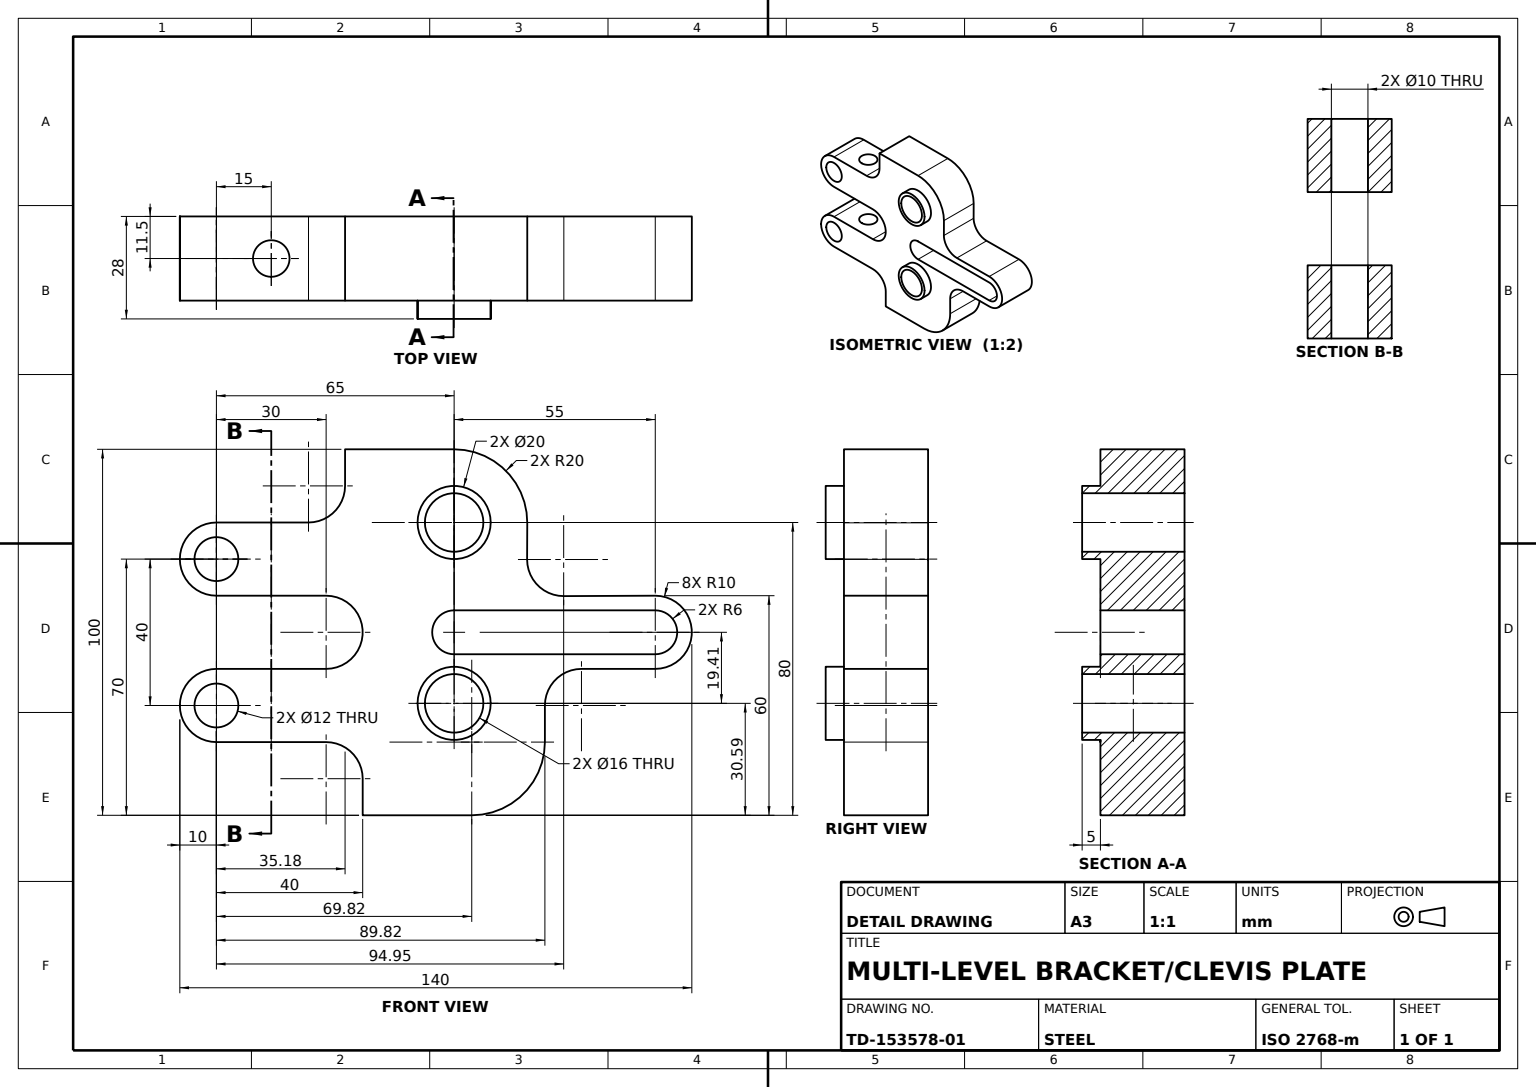
from build123d import *

# Parameters (mm, degrees)
BRACKET_PROFILE_SKETCH_R = 6
BRACKET_BASE_23MM_DEPTH  = 23
BOSS_PAD_SKETCH_R        = 10
BOSS_PAD_SKETCH_R_2      = 8
BOSS_PAD_5MM_DEPTH       = 5
HOLE_10_SKETCH_R         = 5
HOLE_10_DEPTH            = 156.190205877
PROFILE_CUT_SKETCH_R     = 8
PROFILE_CUT_DEPTH        = 150.428912865


with BuildPart() as part:
    # Bracket Profile Sketch → Bracket Base 23mm (new body)
    with BuildSketch(Plane.XY):
        with BuildLine():
            Line((65, -70), (40, -70))
            Line((40, -70), (40, -60))
            ThreePointArc((40, -60), (37.071067812, -52.928932188), (30, -50))
            Line((30, -50), (0, -50))
            ThreePointArc((0, -50), (-10, -40), (0, -30))
            Line((0, -30), (30, -30))
            ThreePointArc((30, -30), (40, -20), (30, -10))
            Line((30, -10), (0, -10))
            ThreePointArc((0, -10), (-10, 0), (0, 10))
            Line((0, 10), (25.18, 10))
            ThreePointArc((25.18, 10), (32.251067812, 12.928932188), (35.18, 20))
            Line((35.18, 20), (35.18, 30))
            Line((35.18, 30), (65, 30))
            ThreePointArc((65, 30), (79.174121887, 24.110280263), (85, 9.910000911))
            Line((85, 9.910000911), (84.955100778, -0.067604024))
            ThreePointArc((84.955100778, -0.067604024), (87.883932045, -7.183671708), (95, -10.112502316))
            Line((95, -10.112502316), (120, -10))
            ThreePointArc((120, -10), (130, -20), (120, -30))
            Line((120, -30), (99.82, -30))
            ThreePointArc((99.82, -30), (92.748932188, -32.928932188), (89.82, -40))
            Line((89.82, -40), (89.82, -50))
            ThreePointArc((89.82, -50), (83.962135624, -64.142135624), (69.82, -70))
            Line((69.82, -70), (65, -70))
        make_face()
        Circle(BRACKET_PROFILE_SKETCH_R, mode=Mode.SUBTRACT)
        with Locations((0, -40)):
            Circle(BRACKET_PROFILE_SKETCH_R, mode=Mode.SUBTRACT)
        with BuildLine():
            Line((120, -26), (65, -26))
            ThreePointArc((65, -26), (59, -20), (65, -14))
            Line((65, -14), (120, -14))
            ThreePointArc((120, -14), (126, -20), (120, -26))
        make_face(mode=Mode.SUBTRACT)
    extrude(amount=BRACKET_BASE_23MM_DEPTH)

    # Boss Pad Sketch → Boss Pad 5mm (add)
    # profile 1 of 2: a face of its own
    with BuildSketch(Plane.XY.offset(23)):
        with Locations((65, 10)):
            Circle(BOSS_PAD_SKETCH_R)
        with Locations((65, 10)):
            Circle(BOSS_PAD_SKETCH_R_2, mode=Mode.SUBTRACT)
    # profile 2 of 2: a face of its own
    with BuildSketch(Plane.XY.offset(23)):
        with Locations((65, -39.411185403)):
            Circle(BOSS_PAD_SKETCH_R)
        with Locations((65, -39.411185403)):
            Circle(BOSS_PAD_SKETCH_R_2, mode=Mode.SUBTRACT)
    extrude(amount=BOSS_PAD_5MM_DEPTH)

    # Hole Ø10 Sketch → Hole Ø10 (cut, through all)
    with BuildSketch(Plane.XZ.offset(50)):
        with Locations(Location((15, 11.5, 0), (0, 0, 270))):
            Circle(HOLE_10_SKETCH_R)
    extrude(amount=-HOLE_10_DEPTH, mode=Mode.SUBTRACT)

    # Profile Cut Sketch → Profile Cut (cut, through all)
    with BuildSketch(Plane.XY.offset(23)):
        with Locations((65, 10)):
            Circle(PROFILE_CUT_SKETCH_R)
        with Locations((65, -39.411185403)):
            Circle(PROFILE_CUT_SKETCH_R)
    extrude(amount=-PROFILE_CUT_DEPTH, mode=Mode.SUBTRACT)


solid = part.part
